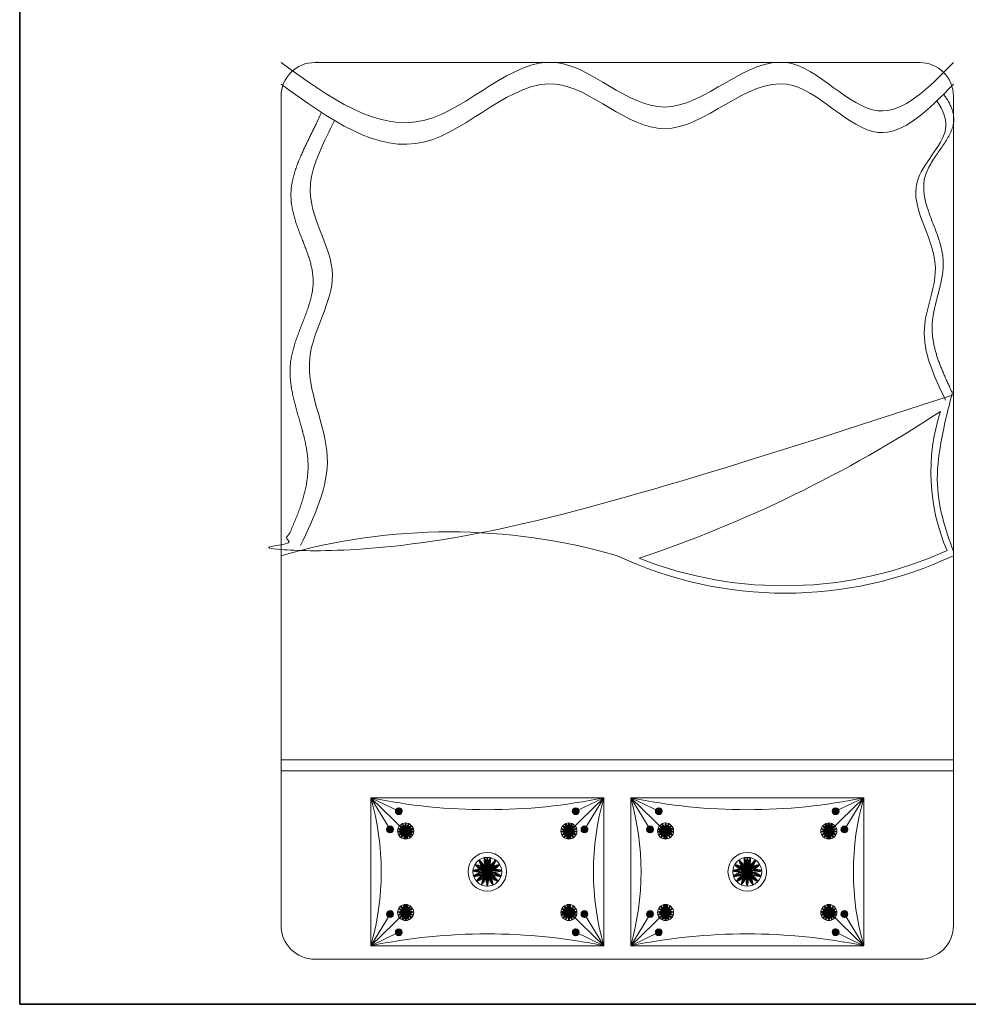
# Model space of a CAD drawing. Units: inches. Extents: x -61 to 1599, y -1316 to 257.
# Tile 158 of 204: x 1066 to 1163, y -1202 to -1101. Entities that reach past the tile are written whole.
import ezdxf

# ---------------------------------------------------------------- set-up
doc = ezdxf.new("R2010")
doc.units = ezdxf.units.IN
doc.header["$MEASUREMENT"] = 0
doc.layers.add('FURNITURE', color=83, linetype='Continuous', lineweight=18)
doc.layers.add('WALLS', color=4, linetype='Continuous', lineweight=35)
doc.layers.add('LT', color=8, linetype='Continuous')

# ---------------------------------------------------------------- blocks, each defined once
blk = doc.blocks.new('*U15')
at = {"layer": 'LT'}
blk.add_line((0, 0.18), (0, -0.18), dxfattribs=at)
for centre, start, end in [((0.51, 0), 160.9983, 199.0017), ((-0.51, 0), 340.9983, 19.0017)]:
    blk.add_arc(centre, 0.539, start, end, dxfattribs=at)
blk = doc.blocks.new('*U16')
at = {"layer": 'LT', "transparency": 16777216}
for p, rotation in [((-66.65, -18.83), 96), ((-66.64, -18.76), 72), ((-66.63, -18.9), 120), ((-66.61, -18.69), 48.00000000000001), ((-66.58, -18.95), 144), ((-66.55, -18.65), 24), ((-66.51, -18.98), 168.0000000000001), ((-66.4, -18.65), 336.0000000000001), ((-66.37, -18.95), 216), ((-66.44, -18.98), 192), ((-66.34, -18.69), 312), ((-66.32, -18.9), 240), ((-66.31, -18.76), 288.0000000000001), ((-66.3, -18.83), 264)]:
    blk.add_blockref('*U15', p, dxfattribs=dict(at, rotation=rotation))
blk.add_blockref('*U15', (-66.48, -18.63), dxfattribs=at)
blk = doc.blocks.new('*U45')
at = {"layer": 'LT'}
blk.add_line((0, 0.18), (0, -0.18), dxfattribs=at)
for centre, start, end in [((0.51, 0), 160.9983, 199.0017), ((-0.51, 0), 340.9983, 19.0017)]:
    blk.add_arc(centre, 0.539, start, end, dxfattribs=at)
blk = doc.blocks.new('*U46')
at = {"layer": 'LT', "transparency": 16777216}
for p, rotation in [((-66.65, -18.83), 96), ((-66.64, -18.76), 72), ((-66.63, -18.9), 120), ((-66.61, -18.69), 48.00000000000001), ((-66.58, -18.95), 144), ((-66.55, -18.65), 24), ((-66.51, -18.98), 168.0000000000001), ((-66.4, -18.65), 336.0000000000001), ((-66.37, -18.95), 216), ((-66.44, -18.98), 192), ((-66.34, -18.69), 312), ((-66.32, -18.9), 240), ((-66.31, -18.76), 288.0000000000001), ((-66.3, -18.83), 264)]:
    blk.add_blockref('*U45', p, dxfattribs=dict(at, rotation=rotation))
blk.add_blockref('*U45', (-66.48, -18.63), dxfattribs=at)
blk = doc.blocks.new('*U9')
at = {"layer": 'LT'}
blk.add_line((0, 0.18), (0, -0.18), dxfattribs=at)
for centre, start, end in [((0.51, 0), 160.9983, 199.0017), ((-0.51, 0), 340.9983, 19.0017)]:
    blk.add_arc(centre, 0.539, start, end, dxfattribs=at)
blk = doc.blocks.new('*U10')
at = {"layer": 'LT', "transparency": 16777216}
for p, rotation in [((-66.65, -18.83), 96), ((-66.64, -18.76), 72), ((-66.63, -18.9), 120), ((-66.61, -18.69), 48.00000000000001), ((-66.58, -18.95), 144), ((-66.55, -18.65), 24), ((-66.51, -18.98), 168.0000000000001), ((-66.4, -18.65), 336.0000000000001), ((-66.37, -18.95), 216), ((-66.44, -18.98), 192), ((-66.34, -18.69), 312), ((-66.32, -18.9), 240), ((-66.31, -18.76), 288.0000000000001), ((-66.3, -18.83), 264)]:
    blk.add_blockref('*U9', p, dxfattribs=dict(at, rotation=rotation))
blk.add_blockref('*U9', (-66.48, -18.63), dxfattribs=at)
blk = doc.blocks.new('*U39')
at = {"layer": 'LT'}
blk.add_line((0, 0.18), (0, -0.18), dxfattribs=at)
for centre, start, end in [((0.51, 0), 160.9983, 199.0017), ((-0.51, 0), 340.9983, 19.0017)]:
    blk.add_arc(centre, 0.539, start, end, dxfattribs=at)
blk = doc.blocks.new('*U40')
at = {"layer": 'LT', "transparency": 16777216}
for p, rotation in [((-66.65, -18.83), 96), ((-66.64, -18.76), 72), ((-66.63, -18.9), 120), ((-66.61, -18.69), 48.00000000000001), ((-66.58, -18.95), 144), ((-66.55, -18.65), 24), ((-66.51, -18.98), 168.0000000000001), ((-66.4, -18.65), 336.0000000000001), ((-66.37, -18.95), 216), ((-66.44, -18.98), 192), ((-66.34, -18.69), 312), ((-66.32, -18.9), 240), ((-66.31, -18.76), 288.0000000000001), ((-66.3, -18.83), 264)]:
    blk.add_blockref('*U39', p, dxfattribs=dict(at, rotation=rotation))
blk.add_blockref('*U39', (-66.48, -18.63), dxfattribs=at)
blk = doc.blocks.new('*U17')
at = {"layer": 'LT'}
blk.add_line((0, 0.41), (0, -0.41), dxfattribs=at)
for centre, start, end in [((1.2, 0), 160.9983, 199.0017), ((-1.2, 0), 340.9983, 19.0017)]:
    blk.add_arc(centre, 1.27, start, end, dxfattribs=at)
blk = doc.blocks.new('*U18')
at = {"layer": 'LT', "transparency": 16777216}
blk.add_blockref('*U17', (-156.33, -43.82), dxfattribs=at)
for p, rotation in [((-156.74, -44.28), 96), ((-156.73, -44.11), 72), ((-156.69, -44.44), 120), ((-156.64, -43.96), 48.00000000000001), ((-156.58, -44.57), 144), ((-156.5, -43.86), 24), ((-156.42, -44.64), 168), ((-156.17, -43.86), 336.0000000000001), ((-156.25, -44.64), 192), ((-156.09, -44.57), 216), ((-156.03, -43.96), 312), ((-155.98, -44.44), 240), ((-155.94, -44.11), 288.0000000000001), ((-155.92, -44.28), 264)]:
    blk.add_blockref('*U17', p, dxfattribs=dict(at, rotation=rotation))
blk = doc.blocks.new('*U33')
at = {"layer": 'LT'}
blk.add_line((0, 0.41), (0, -0.41), dxfattribs=at)
for centre, start, end in [((1.2, 0), 160.9983, 199.0017), ((-1.2, 0), 340.9983, 19.0017)]:
    blk.add_arc(centre, 1.27, start, end, dxfattribs=at)
blk = doc.blocks.new('*U34')
at = {"layer": 'LT', "transparency": 16777216}
blk.add_blockref('*U33', (-156.33, -43.82), dxfattribs=at)
for p, rotation in [((-156.74, -44.28), 96), ((-156.73, -44.11), 72), ((-156.69, -44.44), 120), ((-156.64, -43.96), 48.00000000000001), ((-156.58, -44.57), 144), ((-156.5, -43.86), 24), ((-156.42, -44.64), 168), ((-156.17, -43.86), 336.0000000000001), ((-156.25, -44.64), 192), ((-156.09, -44.57), 216), ((-156.03, -43.96), 312), ((-155.98, -44.44), 240), ((-155.94, -44.11), 288.0000000000001), ((-155.92, -44.28), 264)]:
    blk.add_blockref('*U33', p, dxfattribs=dict(at, rotation=rotation))
blk = doc.blocks.new('*U11')
at = {"layer": 'LT'}
blk.add_line((0, 0.74), (0, -0.74), dxfattribs=at)
for centre, start, end in [((2.15, 0), 160.9983, 199.0017), ((-2.15, 0), 340.9983, 19.0017)]:
    blk.add_arc(centre, 2.27, start, end, dxfattribs=at)
blk = doc.blocks.new('*U12')
at = {"layer": 'LT', "transparency": 16777216}
for p, rotation in [((-280.94, -79.07), 72), ((-280.79, -78.8), 48.00000000000001), ((-280.54, -78.62), 23.99999999999999), ((-279.94, -78.62), 336.0000000000001), ((-279.69, -78.8), 312), ((-279.54, -79.07), 288.0000000000001), ((-280.98, -79.37), 96), ((-280.88, -79.67), 120), ((-280.68, -79.89), 144), ((-280.4, -80.02), 168), ((-280.09, -80.02), 191.9999999999999), ((-279.81, -79.89), 216), ((-279.6, -79.67), 240), ((-279.51, -79.37), 264)]:
    blk.add_blockref('*U11', p, dxfattribs=dict(at, rotation=rotation))
blk.add_blockref('*U11', (-280.24, -78.56), dxfattribs=at)
blk = doc.blocks.new('*U28')
at = {"layer": 'LT'}
blk.add_line((0, 0.41), (0, -0.41), dxfattribs=at)
for centre, start, end in [((1.2, 0), 160.9983, 199.0017), ((-1.2, 0), 340.9983, 19.0017)]:
    blk.add_arc(centre, 1.27, start, end, dxfattribs=at)
blk = doc.blocks.new('*U44')
at = {"layer": 'LT', "transparency": 16777216}
blk.add_blockref('*U28', (-156.33, -43.82), dxfattribs=at)
for p, rotation in [((-156.74, -44.28), 96), ((-156.73, -44.11), 72), ((-156.69, -44.44), 120), ((-156.64, -43.96), 48.00000000000001), ((-156.58, -44.57), 144), ((-156.5, -43.86), 24), ((-156.42, -44.64), 168), ((-156.17, -43.86), 336.0000000000001), ((-156.25, -44.64), 192), ((-156.09, -44.57), 216), ((-156.03, -43.96), 312), ((-155.98, -44.44), 240), ((-155.94, -44.11), 288.0000000000001), ((-155.92, -44.28), 264)]:
    blk.add_blockref('*U28', p, dxfattribs=dict(at, rotation=rotation))
blk = doc.blocks.new('*U13')
at = {"layer": 'LT'}
blk.add_line((0, 0.41), (0, -0.41), dxfattribs=at)
for centre, start, end in [((1.2, 0), 160.9983, 199.0017), ((-1.2, 0), 340.9983, 19.0017)]:
    blk.add_arc(centre, 1.27, start, end, dxfattribs=at)
blk = doc.blocks.new('*U14')
at = {"layer": 'LT', "transparency": 16777216}
blk.add_blockref('*U13', (-156.33, -43.82), dxfattribs=at)
for p, rotation in [((-156.74, -44.28), 96), ((-156.73, -44.11), 72), ((-156.69, -44.44), 120), ((-156.64, -43.96), 48.00000000000001), ((-156.58, -44.57), 144), ((-156.5, -43.86), 24), ((-156.42, -44.64), 168), ((-156.17, -43.86), 336.0000000000001), ((-156.25, -44.64), 192), ((-156.09, -44.57), 216), ((-156.03, -43.96), 312), ((-155.98, -44.44), 240), ((-155.94, -44.11), 288.0000000000001), ((-155.92, -44.28), 264)]:
    blk.add_blockref('*U13', p, dxfattribs=dict(at, rotation=rotation))
blk = doc.blocks.new('*U19')
at = {"layer": 'LT'}
blk.add_line((0, 0.18), (0, -0.18), dxfattribs=at)
for centre, start, end in [((0.51, 0), 160.9983, 199.0017), ((-0.51, 0), 340.9983, 19.0017)]:
    blk.add_arc(centre, 0.539, start, end, dxfattribs=at)
blk = doc.blocks.new('*U6')
at = {"layer": 'LT', "transparency": 16777216}
for p, rotation in [((-66.65, -18.83), 96), ((-66.64, -18.76), 72), ((-66.63, -18.9), 120), ((-66.61, -18.69), 48.00000000000001), ((-66.58, -18.95), 144), ((-66.55, -18.65), 24), ((-66.51, -18.98), 168.0000000000001), ((-66.4, -18.65), 336.0000000000001), ((-66.37, -18.95), 216), ((-66.44, -18.98), 192), ((-66.34, -18.69), 312), ((-66.32, -18.9), 240), ((-66.31, -18.76), 288.0000000000001), ((-66.3, -18.83), 264)]:
    blk.add_blockref('*U19', p, dxfattribs=dict(at, rotation=rotation))
blk.add_blockref('*U19', (-66.48, -18.63), dxfattribs=at)
blk = doc.blocks.new('*U35')
at = {"layer": 'LT'}
blk.add_line((0, 0.18), (0, -0.18), dxfattribs=at)
for centre, start, end in [((0.51, 0), 160.9983, 199.0017), ((-0.51, 0), 340.9983, 19.0017)]:
    blk.add_arc(centre, 0.539, start, end, dxfattribs=at)
blk = doc.blocks.new('*U36')
at = {"layer": 'LT', "transparency": 16777216}
for p, rotation in [((-66.65, -18.83), 96), ((-66.64, -18.76), 72), ((-66.63, -18.9), 120), ((-66.61, -18.69), 48.00000000000001), ((-66.58, -18.95), 144), ((-66.55, -18.65), 24), ((-66.51, -18.98), 168.0000000000001), ((-66.4, -18.65), 336.0000000000001), ((-66.37, -18.95), 216), ((-66.44, -18.98), 192), ((-66.34, -18.69), 312), ((-66.32, -18.9), 240), ((-66.31, -18.76), 288.0000000000001), ((-66.3, -18.83), 264)]:
    blk.add_blockref('*U35', p, dxfattribs=dict(at, rotation=rotation))
blk.add_blockref('*U35', (-66.48, -18.63), dxfattribs=at)
blk = doc.blocks.new('*U7')
at = {"layer": 'LT'}
blk.add_line((0, 0.18), (0, -0.18), dxfattribs=at)
for centre, start, end in [((0.51, 0), 160.9983, 199.0017), ((-0.51, 0), 340.9983, 19.0017)]:
    blk.add_arc(centre, 0.539, start, end, dxfattribs=at)
blk = doc.blocks.new('*U8')
at = {"layer": 'LT', "transparency": 16777216}
for p, rotation in [((-66.65, -18.83), 96), ((-66.64, -18.76), 72), ((-66.63, -18.9), 120), ((-66.61, -18.69), 48.00000000000001), ((-66.58, -18.95), 144), ((-66.55, -18.65), 24), ((-66.51, -18.98), 168.0000000000001), ((-66.4, -18.65), 336.0000000000001), ((-66.37, -18.95), 216), ((-66.44, -18.98), 192), ((-66.34, -18.69), 312), ((-66.32, -18.9), 240), ((-66.31, -18.76), 288.0000000000001), ((-66.3, -18.83), 264)]:
    blk.add_blockref('*U7', p, dxfattribs=dict(at, rotation=rotation))
blk.add_blockref('*U7', (-66.48, -18.63), dxfattribs=at)
blk = doc.blocks.new('*U37')
at = {"layer": 'LT'}
blk.add_line((0, 0.18), (0, -0.18), dxfattribs=at)
for centre, start, end in [((0.51, 0), 160.9983, 199.0017), ((-0.51, 0), 340.9983, 19.0017)]:
    blk.add_arc(centre, 0.539, start, end, dxfattribs=at)
blk = doc.blocks.new('*U38')
at = {"layer": 'LT', "transparency": 16777216}
for p, rotation in [((-66.65, -18.83), 96), ((-66.64, -18.76), 72), ((-66.63, -18.9), 120), ((-66.61, -18.69), 48.00000000000001), ((-66.58, -18.95), 144), ((-66.55, -18.65), 24), ((-66.51, -18.98), 168.0000000000001), ((-66.4, -18.65), 336.0000000000001), ((-66.37, -18.95), 216), ((-66.44, -18.98), 192), ((-66.34, -18.69), 312), ((-66.32, -18.9), 240), ((-66.31, -18.76), 288.0000000000001), ((-66.3, -18.83), 264)]:
    blk.add_blockref('*U37', p, dxfattribs=dict(at, rotation=rotation))
blk.add_blockref('*U37', (-66.48, -18.63), dxfattribs=at)
blk = doc.blocks.new('*U3')
at = {"layer": 'LT'}
blk.add_line((0, 0.18), (0, -0.18), dxfattribs=at)
for centre, start, end in [((0.51, 0), 160.9983, 199.0017), ((-0.51, 0), 340.9983, 19.0017)]:
    blk.add_arc(centre, 0.539, start, end, dxfattribs=at)
blk = doc.blocks.new('*U4')
at = {"layer": 'LT', "transparency": 16777216}
for p, rotation in [((-66.65, -18.83), 96), ((-66.64, -18.76), 72), ((-66.63, -18.9), 120), ((-66.61, -18.69), 48.00000000000001), ((-66.58, -18.95), 144), ((-66.55, -18.65), 24), ((-66.51, -18.98), 168.0000000000001), ((-66.4, -18.65), 336.0000000000001), ((-66.37, -18.95), 216), ((-66.44, -18.98), 192), ((-66.34, -18.69), 312), ((-66.32, -18.9), 240), ((-66.31, -18.76), 288.0000000000001), ((-66.3, -18.83), 264)]:
    blk.add_blockref('*U3', p, dxfattribs=dict(at, rotation=rotation))
blk.add_blockref('*U3', (-66.48, -18.63), dxfattribs=at)
blk = doc.blocks.new('*U20')
at = {"layer": 'LT'}
blk.add_line((0, 0.18), (0, -0.18), dxfattribs=at)
for centre, start, end in [((0.51, 0), 160.9983, 199.0017), ((-0.51, 0), 340.9983, 19.0017)]:
    blk.add_arc(centre, 0.539, start, end, dxfattribs=at)
blk = doc.blocks.new('*U21')
at = {"layer": 'LT', "transparency": 16777216}
for p, rotation in [((-66.65, -18.83), 96), ((-66.64, -18.76), 72), ((-66.63, -18.9), 120), ((-66.61, -18.69), 48.00000000000001), ((-66.58, -18.95), 144), ((-66.55, -18.65), 24), ((-66.51, -18.98), 168.0000000000001), ((-66.4, -18.65), 336.0000000000001), ((-66.37, -18.95), 216), ((-66.44, -18.98), 192), ((-66.34, -18.69), 312), ((-66.32, -18.9), 240), ((-66.31, -18.76), 288.0000000000001), ((-66.3, -18.83), 264)]:
    blk.add_blockref('*U20', p, dxfattribs=dict(at, rotation=rotation))
blk.add_blockref('*U20', (-66.48, -18.63), dxfattribs=at)
blk = doc.blocks.new('*U52')
at = {"layer": 'LT'}
blk.add_line((0, 0.18), (0, -0.18), dxfattribs=at)
for centre, start, end in [((0.51, 0), 160.9983, 199.0017), ((-0.51, 0), 340.9983, 19.0017)]:
    blk.add_arc(centre, 0.539, start, end, dxfattribs=at)
blk = doc.blocks.new('*U53')
at = {"layer": 'LT', "transparency": 16777216}
for p, rotation in [((-66.65, -18.83), 96), ((-66.64, -18.76), 72), ((-66.63, -18.9), 120), ((-66.61, -18.69), 48.00000000000001), ((-66.58, -18.95), 144), ((-66.55, -18.65), 24), ((-66.51, -18.98), 168.0000000000001), ((-66.4, -18.65), 336.0000000000001), ((-66.37, -18.95), 216), ((-66.44, -18.98), 192), ((-66.34, -18.69), 312), ((-66.32, -18.9), 240), ((-66.31, -18.76), 288.0000000000001), ((-66.3, -18.83), 264)]:
    blk.add_blockref('*U52', p, dxfattribs=dict(at, rotation=rotation))
blk.add_blockref('*U52', (-66.48, -18.63), dxfattribs=at)
blk = doc.blocks.new('*U29')
at = {"layer": 'LT'}
blk.add_line((0, 0.18), (0, -0.18), dxfattribs=at)
for centre, start, end in [((0.51, 0), 160.9983, 199.0017), ((-0.51, 0), 340.9983, 19.0017)]:
    blk.add_arc(centre, 0.539, start, end, dxfattribs=at)
blk = doc.blocks.new('*U30')
at = {"layer": 'LT', "transparency": 16777216}
for p, rotation in [((-66.65, -18.83), 96), ((-66.64, -18.76), 72), ((-66.63, -18.9), 120), ((-66.61, -18.69), 48.00000000000001), ((-66.58, -18.95), 144), ((-66.55, -18.65), 24), ((-66.51, -18.98), 168.0000000000001), ((-66.4, -18.65), 336.0000000000001), ((-66.37, -18.95), 216), ((-66.44, -18.98), 192), ((-66.34, -18.69), 312), ((-66.32, -18.9), 240), ((-66.31, -18.76), 288.0000000000001), ((-66.3, -18.83), 264)]:
    blk.add_blockref('*U29', p, dxfattribs=dict(at, rotation=rotation))
blk.add_blockref('*U29', (-66.48, -18.63), dxfattribs=at)
blk = doc.blocks.new('*U5')
at = {"layer": 'LT'}
blk.add_line((0, 0.41), (0, -0.41), dxfattribs=at)
for centre, start, end in [((1.2, 0), 160.9983, 199.0017), ((-1.2, 0), 340.9983, 19.0017)]:
    blk.add_arc(centre, 1.27, start, end, dxfattribs=at)
blk = doc.blocks.new('*U47')
at = {"layer": 'LT', "transparency": 16777216}
blk.add_blockref('*U5', (-156.33, -43.82), dxfattribs=at)
for p, rotation in [((-156.74, -44.28), 96), ((-156.73, -44.11), 72), ((-156.69, -44.44), 120), ((-156.64, -43.96), 48.00000000000001), ((-156.58, -44.57), 144), ((-156.5, -43.86), 24), ((-156.42, -44.64), 168), ((-156.17, -43.86), 336.0000000000001), ((-156.25, -44.64), 192), ((-156.09, -44.57), 216), ((-156.03, -43.96), 312), ((-155.98, -44.44), 240), ((-155.94, -44.11), 288.0000000000001), ((-155.92, -44.28), 264)]:
    blk.add_blockref('*U5', p, dxfattribs=dict(at, rotation=rotation))
blk = doc.blocks.new('*U22')
at = {"layer": 'LT'}
blk.add_line((0, 0.41), (0, -0.41), dxfattribs=at)
for centre, start, end in [((1.2, 0), 160.9983, 199.0017), ((-1.2, 0), 340.9983, 19.0017)]:
    blk.add_arc(centre, 1.27, start, end, dxfattribs=at)
blk = doc.blocks.new('*U23')
at = {"layer": 'LT', "transparency": 16777216}
blk.add_blockref('*U22', (-156.33, -43.82), dxfattribs=at)
for p, rotation in [((-156.74, -44.28), 96), ((-156.73, -44.11), 72), ((-156.69, -44.44), 120), ((-156.64, -43.96), 48.00000000000001), ((-156.58, -44.57), 144), ((-156.5, -43.86), 24), ((-156.42, -44.64), 168), ((-156.17, -43.86), 336.0000000000001), ((-156.25, -44.64), 192), ((-156.09, -44.57), 216), ((-156.03, -43.96), 312), ((-155.98, -44.44), 240), ((-155.94, -44.11), 288.0000000000001), ((-155.92, -44.28), 264)]:
    blk.add_blockref('*U22', p, dxfattribs=dict(at, rotation=rotation))
blk = doc.blocks.new('*U54')
at = {"layer": 'LT'}
blk.add_line((0, 0.74), (0, -0.74), dxfattribs=at)
for centre, start, end in [((2.15, 0), 160.9983, 199.0017), ((-2.15, 0), 340.9983, 19.0017)]:
    blk.add_arc(centre, 2.27, start, end, dxfattribs=at)
blk = doc.blocks.new('*U41')
at = {"layer": 'LT', "transparency": 16777216}
for p, rotation in [((-280.94, -79.07), 72), ((-280.79, -78.8), 48.00000000000001), ((-280.54, -78.62), 23.99999999999999), ((-279.94, -78.62), 336.0000000000001), ((-279.69, -78.8), 312), ((-279.54, -79.07), 288.0000000000001), ((-280.98, -79.37), 96), ((-280.88, -79.67), 120), ((-280.68, -79.89), 144), ((-280.4, -80.02), 168), ((-280.09, -80.02), 191.9999999999999), ((-279.81, -79.89), 216), ((-279.6, -79.67), 240), ((-279.51, -79.37), 264)]:
    blk.add_blockref('*U54', p, dxfattribs=dict(at, rotation=rotation))
blk.add_blockref('*U54', (-280.24, -78.56), dxfattribs=at)
blk = doc.blocks.new('*U42')
at = {"layer": 'LT'}
blk.add_line((0, 0.41), (0, -0.41), dxfattribs=at)
for centre, start, end in [((1.2, 0), 160.9983, 199.0017), ((-1.2, 0), 340.9983, 19.0017)]:
    blk.add_arc(centre, 1.27, start, end, dxfattribs=at)
blk = doc.blocks.new('*U43')
at = {"layer": 'LT', "transparency": 16777216}
blk.add_blockref('*U42', (-156.33, -43.82), dxfattribs=at)
for p, rotation in [((-156.74, -44.28), 96), ((-156.73, -44.11), 72), ((-156.69, -44.44), 120), ((-156.64, -43.96), 48.00000000000001), ((-156.58, -44.57), 144), ((-156.5, -43.86), 24), ((-156.42, -44.64), 168), ((-156.17, -43.86), 336.0000000000001), ((-156.25, -44.64), 192), ((-156.09, -44.57), 216), ((-156.03, -43.96), 312), ((-155.98, -44.44), 240), ((-155.94, -44.11), 288.0000000000001), ((-155.92, -44.28), 264)]:
    blk.add_blockref('*U42', p, dxfattribs=dict(at, rotation=rotation))
blk = doc.blocks.new('*U31')
at = {"layer": 'LT'}
blk.add_line((0, 0.41), (0, -0.41), dxfattribs=at)
for centre, start, end in [((1.2, 0), 160.9983, 199.0017), ((-1.2, 0), 340.9983, 19.0017)]:
    blk.add_arc(centre, 1.27, start, end, dxfattribs=at)
blk = doc.blocks.new('*U32')
at = {"layer": 'LT', "transparency": 16777216}
blk.add_blockref('*U31', (-156.33, -43.82), dxfattribs=at)
for p, rotation in [((-156.74, -44.28), 96), ((-156.73, -44.11), 72), ((-156.69, -44.44), 120), ((-156.64, -43.96), 48.00000000000001), ((-156.58, -44.57), 144), ((-156.5, -43.86), 24), ((-156.42, -44.64), 168), ((-156.17, -43.86), 336.0000000000001), ((-156.25, -44.64), 192), ((-156.09, -44.57), 216), ((-156.03, -43.96), 312), ((-155.98, -44.44), 240), ((-155.94, -44.11), 288.0000000000001), ((-155.92, -44.28), 264)]:
    blk.add_blockref('*U31', p, dxfattribs=dict(at, rotation=rotation))
blk = doc.blocks.new('*U48')
at = {"layer": 'LT'}
blk.add_line((0, 0.18), (0, -0.18), dxfattribs=at)
for centre, start, end in [((0.51, 0), 160.9983, 199.0017), ((-0.51, 0), 340.9983, 19.0017)]:
    blk.add_arc(centre, 0.539, start, end, dxfattribs=at)
blk = doc.blocks.new('*U49')
at = {"layer": 'LT', "transparency": 16777216}
for p, rotation in [((-66.65, -18.83), 96), ((-66.64, -18.76), 72), ((-66.63, -18.9), 120), ((-66.61, -18.69), 48.00000000000001), ((-66.58, -18.95), 144), ((-66.55, -18.65), 24), ((-66.51, -18.98), 168.0000000000001), ((-66.4, -18.65), 336.0000000000001), ((-66.37, -18.95), 216), ((-66.44, -18.98), 192), ((-66.34, -18.69), 312), ((-66.32, -18.9), 240), ((-66.31, -18.76), 288.0000000000001), ((-66.3, -18.83), 264)]:
    blk.add_blockref('*U48', p, dxfattribs=dict(at, rotation=rotation))
blk.add_blockref('*U48', (-66.48, -18.63), dxfattribs=at)
blk = doc.blocks.new('*U24')
at = {"layer": 'LT'}
blk.add_line((0, 0.18), (0, -0.18), dxfattribs=at)
for centre, start, end in [((0.51, 0), 160.9983, 199.0017), ((-0.51, 0), 340.9983, 19.0017)]:
    blk.add_arc(centre, 0.539, start, end, dxfattribs=at)
blk = doc.blocks.new('*U25')
at = {"layer": 'LT', "transparency": 16777216}
for p, rotation in [((-66.65, -18.83), 96), ((-66.64, -18.76), 72), ((-66.63, -18.9), 120), ((-66.61, -18.69), 48.00000000000001), ((-66.58, -18.95), 144), ((-66.55, -18.65), 24), ((-66.51, -18.98), 168.0000000000001), ((-66.4, -18.65), 336.0000000000001), ((-66.37, -18.95), 216), ((-66.44, -18.98), 192), ((-66.34, -18.69), 312), ((-66.32, -18.9), 240), ((-66.31, -18.76), 288.0000000000001), ((-66.3, -18.83), 264)]:
    blk.add_blockref('*U24', p, dxfattribs=dict(at, rotation=rotation))
blk.add_blockref('*U24', (-66.48, -18.63), dxfattribs=at)
blk = doc.blocks.new('*U50')
at = {"layer": 'LT'}
blk.add_line((0, 0.18), (0, -0.18), dxfattribs=at)
for centre, start, end in [((0.51, 0), 160.9983, 199.0017), ((-0.51, 0), 340.9983, 19.0017)]:
    blk.add_arc(centre, 0.539, start, end, dxfattribs=at)
blk = doc.blocks.new('*U51')
at = {"layer": 'LT', "transparency": 16777216}
for p, rotation in [((-66.65, -18.83), 96), ((-66.64, -18.76), 72), ((-66.63, -18.9), 120), ((-66.61, -18.69), 48.00000000000001), ((-66.58, -18.95), 144), ((-66.55, -18.65), 24), ((-66.51, -18.98), 168.0000000000001), ((-66.4, -18.65), 336.0000000000001), ((-66.37, -18.95), 216), ((-66.44, -18.98), 192), ((-66.34, -18.69), 312), ((-66.32, -18.9), 240), ((-66.31, -18.76), 288.0000000000001), ((-66.3, -18.83), 264)]:
    blk.add_blockref('*U50', p, dxfattribs=dict(at, rotation=rotation))
blk.add_blockref('*U50', (-66.48, -18.63), dxfattribs=at)
blk = doc.blocks.new('*U26')
at = {"layer": 'LT'}
blk.add_line((0, 0.18), (0, -0.18), dxfattribs=at)
for centre, start, end in [((0.51, 0), 160.9983, 199.0017), ((-0.51, 0), 340.9983, 19.0017)]:
    blk.add_arc(centre, 0.539, start, end, dxfattribs=at)
blk = doc.blocks.new('*U27')
at = {"layer": 'LT', "transparency": 16777216}
for p, rotation in [((-66.65, -18.83), 96), ((-66.64, -18.76), 72), ((-66.63, -18.9), 120), ((-66.61, -18.69), 48.00000000000001), ((-66.58, -18.95), 144), ((-66.55, -18.65), 24), ((-66.51, -18.98), 168.0000000000001), ((-66.4, -18.65), 336.0000000000001), ((-66.37, -18.95), 216), ((-66.44, -18.98), 192), ((-66.34, -18.69), 312), ((-66.32, -18.9), 240), ((-66.31, -18.76), 288.0000000000001), ((-66.3, -18.83), 264)]:
    blk.add_blockref('*U26', p, dxfattribs=dict(at, rotation=rotation))
blk.add_blockref('*U26', (-66.48, -18.63), dxfattribs=at)
blk = doc.blocks.new('BED-DOUBLE')
for p, q in [((1.27, 20.47), (70.26, 20.47)), ((1.27, 19.32), (70.26, 19.32)), ((10.47, 1.38), (10.47, 16.56)), ((34.39, 16.56), (10.47, 16.56)), ((10.47, 16.56), (13.35, 15.18)), ((10.47, 16.56), (14.04, 13.11)), ((10.47, 16.56), (12.45, 13.31)), ((34.39, 16.56), (30.82, 13.11)), ((34.39, 16.56), (31.51, 15.18)), ((34.39, 16.56), (32.4, 13.31)), ((37.15, 1.38), (37.15, 16.56)), ((61.06, 16.56), (37.15, 16.56)), ((37.15, 16.56), (40.03, 15.18)), ((37.15, 16.56), (40.71, 13.11)), ((37.15, 16.56), (39.13, 13.31)), ((61.06, 16.56), (57.5, 13.11)), ((61.06, 16.56), (58.18, 15.18)), ((61.06, 16.56), (59.08, 13.31)), ((13.35, 15.18), (13.35, 14.83)), ((31.51, 15.18), (31.51, 14.83)), ((40.03, 15.18), (40.03, 14.83)), ((58.18, 15.18), (58.18, 14.83)), ((12.45, 13.31), (12.45, 12.95)), ((14.05, 13.15), (14.05, 12.32)), ((30.81, 13.15), (30.81, 12.32)), ((32.4, 13.31), (32.4, 12.95)), ((39.13, 13.31), (39.13, 12.95)), ((40.73, 13.15), (40.73, 12.32)), ((57.48, 13.15), (57.48, 12.32)), ((59.08, 13.31), (59.08, 12.95)), ((22.43, 8.97), (22.43, 10.45)), ((49.11, 8.97), (49.11, 10.45)), ((14.05, 4.79), (14.05, 5.61)), ((30.81, 4.79), (30.81, 5.61)), ((40.73, 4.79), (40.73, 5.61)), ((57.48, 4.79), (57.48, 5.61)), ((10.47, 1.38), (14.04, 4.83)), ((10.47, 1.38), (12.45, 4.63)), ((12.45, 4.63), (12.45, 4.98)), ((34.39, 1.38), (30.82, 4.83)), ((32.4, 4.63), (32.4, 4.98)), ((34.39, 1.38), (32.4, 4.63)), ((37.15, 1.38), (40.71, 4.83)), ((37.15, 1.38), (39.13, 4.63)), ((39.13, 4.63), (39.13, 4.98)), ((61.06, 1.38), (57.5, 4.83)), ((59.08, 4.63), (59.08, 4.98)), ((61.06, 1.38), (59.08, 4.63)), ((13.35, 2.76), (13.35, 3.11)), ((31.51, 2.76), (31.51, 3.11)), ((40.03, 2.76), (40.03, 3.11)), ((58.18, 2.76), (58.18, 3.11)), ((10.47, 1.38), (13.35, 2.76)), ((34.39, 1.38), (31.51, 2.76)), ((37.15, 1.38), (40.03, 2.76)), ((61.06, 1.38), (58.18, 2.76)), ((34.39, 1.38), (34.39, 1.38)), ((61.06, 1.38), (61.06, 1.38))]:
    blk.add_line(p, q)
for points in [[(1.27, 88.54), (1.27, 3.45, 0.414214), (4.72, 0), (66.81, 0, 0.414214), (70.26, 3.45), (70.26, 88.54, 0.414214), (66.81, 91.99), (4.72, 91.99, 0.414214)], [(38.01, 41.13, 0.064396), (68.93, 56.18, 0.181766), (69.61, 41.92, -0.202767)], [(13.35, 15.18, 0.167358), (13.35, 14.83, 0.167358)], [(40.03, 15.18, 0.167358), (40.03, 14.83, 0.167358)], [(12.45, 13.31, 0.167358), (12.45, 12.95, 0.167358)], [(14.05, 13.15, 0.167358), (14.05, 12.32, 0.167358)], [(30.81, 12.32, 0.167358), (30.81, 13.15, 0.167358)], [(32.4, 12.95, 0.167358), (32.4, 13.31, 0.167358)], [(39.13, 13.31, 0.167358), (39.13, 12.95, 0.167358)], [(40.73, 13.15, 0.167358), (40.73, 12.32, 0.167358)], [(57.48, 12.32, 0.167358), (57.48, 13.15, 0.167358)], [(59.08, 12.95, 0.167358), (59.08, 13.31, 0.167358)], [(22.43, 8.97, 0.167358), (22.43, 10.45, 0.167358)], [(49.11, 8.97, 0.167358), (49.11, 10.45, 0.167358)], [(14.05, 5.61, 0.167358), (14.05, 4.79, 0.167358)], [(30.81, 4.79, 0.167358), (30.81, 5.61, 0.167358)], [(40.73, 5.61, 0.167358), (40.73, 4.79, 0.167358)], [(57.48, 4.79, 0.167358), (57.48, 5.61, 0.167358)], [(12.45, 4.98, 0.167358), (12.45, 4.63, 0.167358)], [(32.4, 4.63, 0.167358), (32.4, 4.98, 0.167358)], [(39.13, 4.98, 0.167358), (39.13, 4.63, 0.167358)], [(59.08, 4.63, 0.167358), (59.08, 4.98, 0.167358)], [(13.35, 3.11, 0.167358), (13.35, 2.76, 0.167358)], [(31.51, 2.76, 0.167358), (31.51, 3.11, 0.167358)], [(40.03, 3.11, 0.167358), (40.03, 2.76, 0.167358)], [(58.18, 2.76, 0.167358), (58.18, 3.11, 0.167358)]]:
    blk.add_lwpolyline(points, format="xyb", close=True)
blk.add_lwpolyline([(70.26, 41.39, -0.22309), (35.77, 41.39, 0.142156), (1.27, 41.39)], format="xyb")
for points in [[(34.39, 16.56), (34.39, 1.38), (10.47, 1.38), (10.47, 16.56), (34.39, 16.56), (34.39, 1.38), (10.47, 1.38)], [(61.06, 16.56), (61.06, 1.38), (37.15, 1.38)]]:
    blk.add_lwpolyline(points)
for centre, radius in [((13.35, 15.18), 0.351), ((31.51, 15.18), 0.351), ((40.03, 15.18), 0.351), ((58.18, 15.18), 0.351), ((12.45, 13.31), 0.351), ((14.05, 13.15), 0.825), ((30.81, 13.15), 0.825), ((32.4, 13.31), 0.351), ((39.13, 13.31), 0.351), ((40.73, 13.15), 0.825), ((57.48, 13.15), 0.825), ((59.08, 13.31), 0.351), ((22.43, 8.97), 1.98), ((22.43, 8.97), 1.48), ((49.11, 8.97), 1.98), ((49.11, 8.97), 1.48), ((14.05, 4.79), 0.825), ((30.81, 4.79), 0.825), ((40.73, 4.79), 0.825), ((57.48, 4.79), 0.825), ((12.45, 4.63), 0.351), ((32.4, 4.63), 0.351), ((39.13, 4.63), 0.351), ((59.08, 4.63), 0.351), ((13.35, 2.76), 0.351), ((31.51, 2.76), 0.351), ((40.03, 2.76), 0.351), ((58.18, 2.76), 0.351)]:
    blk.add_circle(centre, radius)
for centre, radius, start, end in [((-16, 8.97), 27.54, 344.0046, 15.9954), ((22.43, 74.54), 59.2, 258.3468, 281.6532), ((60.86, 8.97), 27.54, 164.0046, 195.9954), ((10.67, 8.97), 27.54, 344.0046, 15.9954), ((49.11, 74.54), 59.2, 258.3468, 281.6532), ((87.54, 8.97), 27.54, 164.0046, 195.9954), ((32.02, 15), 0.539, 160.9983, 199.0017), ((31, 15), 0.539, 340.9983, 19.0017), ((58.69, 15), 0.539, 160.9983, 199.0017), ((57.68, 15), 0.539, 340.9983, 19.0017), ((22.43, -56.6), 59.2, 78.3468, 101.6532), ((49.11, -56.6), 59.2, 78.3468, 101.6532)]:
    blk.add_arc(centre, radius, start, end)
for points, knots in [([(70.26, 91.99), (67.71, 89.38), (62.21, 83.76), (52.49, 96.72), (40.92, 82.74), (28.61, 96.74), (15.69, 81.53), (6.21, 88.41), (1.27, 91.99)], [0, 0, 0, 0, 9.176033, 19.753992, 33.150145, 45.209422, 59.881559, 75.764594, 75.764594, 75.764594, 75.764594]), ([(70.26, 89.76), (67.71, 87.16), (62.21, 81.54), (52.49, 94.5), (40.92, 80.52), (28.61, 94.52), (15.69, 79.31), (6.21, 86.19), (1.27, 89.76)], [0, 0, 0, 0, 9.176033, 19.753992, 33.150145, 45.209422, 59.881559, 75.764594, 75.764594, 75.764594, 75.764594]), ([(69.45, 57.36), (68.29, 59.79), (66.11, 64.34), (70.04, 71.91), (64.12, 79.11), (70.31, 84.4), (69.24, 87.09), (68.55, 88.05)], [0, 0, 0, 0, 6.649676, 12.451782, 19.973966, 25.324174, 28.349676, 28.349676, 28.349676, 28.349676]), ([(3.25, 42.44), (4.7, 45.45), (7.72, 51.72), (2.12, 61.25), (8.81, 70.52), (2.43, 77.93), (5.72, 83.91), (6.75, 86.04)], [0, 0, 0, 0, 8.27671, 17.241866, 24.903358, 33.244933, 38.427294, 38.427294, 38.427294, 38.427294])]:
    blk.add_open_spline(points, degree=3, knots=knots)
blk.add_open_spline([(5.01, 91.99), (4.99, 92.01), (4.96, 92.03), (4.94, 92.04)], degree=3)
for points, weights, knots in [([(70.26, 41.83), (68.02, 47.03), (68.02, 52.7), (70.26, 57.9), (69.1, 60.33), (66.92, 64.87), (70.85, 72.44), (64.93, 79.65), (71.19, 84.99), (70.01, 87.73), (69.25, 88.74)], [1, 0.945466318698, 0.945466318698, 1, 1, 1, 1, 1, 1, 1, 1], [0, 0, 0, 0, 0.814571, 0.814571, 0.814571, 7.464247, 13.266353, 20.788537, 26.138745, 29.321895, 29.321895, 29.321895, 29.321895]), ([(70.26, 57.9), (59.86, 50.94), (48.6, 45.5), (36.68, 41.68), (36.46, 41.77), (36.25, 41.87), (36.03, 41.97), (24.6, 45.28), (12.69, 45.26), (1.27, 41.89), (2.72, 44.9), (5.74, 51.17), (0.14, 60.7), (6.83, 69.97), (0.11, 77.79), (4.35, 84.38), (5.4, 86.88)], [1, 0.993520320424, 0.993520320424, 1, 0.99997444972, 0.99997444972, 1, 0.973174868659, 0.973174868659, 1, 1, 1, 1, 1, 1, 1, 1], [0, 0, 0, 0, 0.279074, 0.279074, 0.279074, 0.296584, 0.296584, 0.296584, 0.865868, 0.865868, 0.865868, 9.142578, 18.107734, 25.769226, 34.110801, 40.441511, 40.441511, 40.441511, 40.441511])]:
    blk.add_rational_spline(points, weights, degree=3, knots=knots)
for name, p in [('*U40', (79.83, 33.99)), ('*U30', (106.5, 33.99)), ('*U46', (78.93, 32.11)), ('*U34', (170.39, 57.38)), ('*U21', (105.61, 32.11)), ('*U23', (197.06, 57.38))]:
    blk.add_blockref(name, p)
at = {"extrusion": (0, 0, -1), "zscale": -1}
for name, p in [('*U36', (34.97, 33.99)), ('*U25', (8.29, 33.99)), ('*U14', (125.53, 57.38)), ('*U38', (34.07, 32.11)), ('*U32', (98.85, 57.38)), ('*U27', (7.39, 32.11))]:
    blk.add_blockref(name, p, dxfattribs=at)
at = {"rotation": 180}
for name, p in [('*U12', (-257.81, -70.33)), ('*U41', (-231.14, -70.33)), ('*U44', (-125.53, -39.45)), ('*U43', (-98.85, -39.45)), ('*U8', (-34.07, -14.18)), ('*U51', (-7.39, -14.18)), ('*U6', (-34.97, -16.05)), ('*U49', (-8.29, -16.05))]:
    blk.add_blockref(name, p, dxfattribs=at)
at = {"extrusion": (0, 0, -1), "zscale": -1, "rotation": 180}
for name, p in [('*U18', (-170.39, -39.45)), ('*U47', (-197.06, -39.45)), ('*U16', (-78.93, -14.18)), ('*U4', (-105.61, -14.18)), ('*U10', (-79.83, -16.05)), ('*U53', (-106.5, -16.05))]:
    blk.add_blockref(name, p, dxfattribs=at)

msp = doc.modelspace()

# ---------------------------------------------------------------- linework, layer by layer
at = {"layer": 'WALLS'}
for p, q in [((1065.7028, -1058.169), (1065.7028, -1202.169)), ((1065.7028, -1202.169), (1215.7028, -1202.169))]:
    msp.add_line(p, q, dxfattribs=at)

# ---------------------------------------------------------------- block references
at = {"layer": 'FURNITURE'}
msp.add_blockref('BED-DOUBLE', (1091.2612, -1197.5422), dxfattribs=at)

doc.saveas('drawing.dxf')
